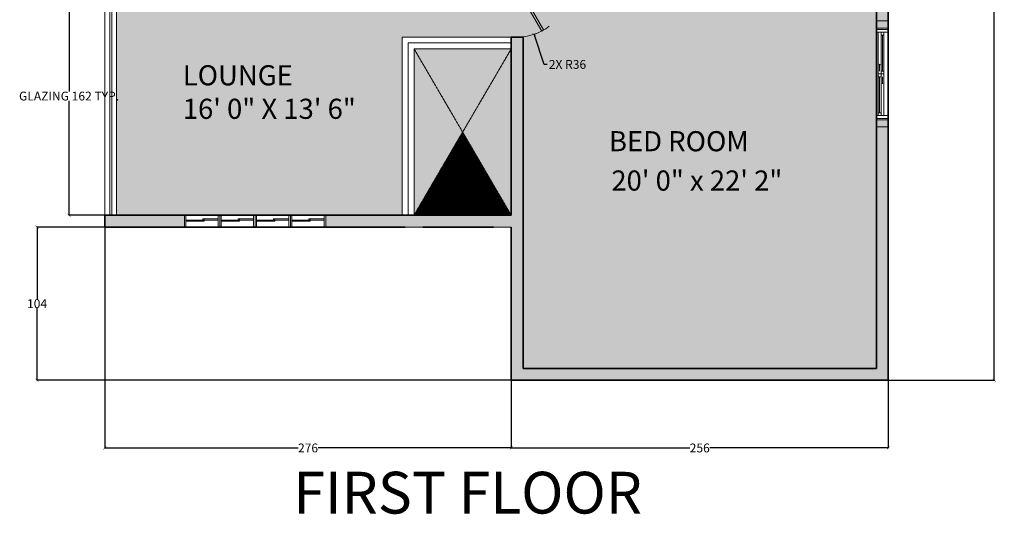
# Model space of a CAD drawing. Units: inches. Extents: x 1704 to 6393, y -157 to 1172.
# Tile 117 of 122: x 4377 to 5046, y 47 to 382. Entities that reach past the tile are written whole.
import ezdxf

# ---------------------------------------------------------------- set-up
doc = ezdxf.new("R2010")
doc.units = ezdxf.units.IN
doc.header["$MEASUREMENT"] = 0
doc.linetypes.add('ACAD_ISO02W100', pattern=[15, 12, -3])
doc.linetypes.add('HIDDEN', pattern=[0.375, 0.25, -0.125])
for name, color, linetype, lineweight in [('A-ANNO-DIMS', 7, 'Continuous', 13), ('A-ANNO-TEXT', 7, 'Continuous', 25), ('A-AREA-IDEN', 7, 'Continuous', 18), ('A-FLOR-OPEN-HIDN', 8, 'HIDDEN', 13), ('A-WALL-OVHD', 8, 'ACAD_ISO02W100', 13), ('A-WALL-PATT', 7, 'Continuous', 13), ('DOORS', 160, 'Continuous', 18), ('GLASS PANEL FASADE', 4, 'Continuous', 18), ('WALLS', 7, 'Continuous', 35), ('WINDOWS', 2, 'Continuous', 18)]:
    doc.layers.add(name, color=color, linetype=linetype, lineweight=lineweight)
doc.layers.add('A-FLOR-PATT', color=7, linetype='Continuous', lineweight=13, true_color=0xf2f2f2)
doc.styles.get("Standard").update_dxf_attribs({"font": 'arial.ttf'})
doc.dimstyles.get("Standard").update_dxf_attribs({"dimtxt": 6, "dimasz": 2, "dimexe": 0.18, "dimexo": 0.0625, "dimgap": 0.09, "dimtad": 0, "dimtih": 1, "dimtoh": 1, "dimdec": 1, "dimzin": 0, "dimdsep": 46, "dimlunit": 3, "dimtxsty": 'Standard', "dimblk": 'ARCHTICK', "dimcen": 0.09, "dimadec": 0, "dimazin": 0, "dimtfac": 1, "dimtdec": 1, "dimtofl": 0, "dimtmove": 0, "dimatfit": 3, "dimfxl": 1, "dimtolj": 1, "dimtzin": 0, "dimarcsym": 0})

# ---------------------------------------------------------------- blocks, each defined once
blk = doc.blocks.new('Door - Left Hung 36 in.')
blk.add_lwpolyline([(0.75, -1.3), (0, 0), (31.18, 18), (31.93, 16.7)], close=True)
blk.add_arc((0, 0), 36, 0, 37.31013)
blk = doc.blocks.new('WIN-SLIDER-72')
for p, q in [((0, 72), (0, 0)), ((0, 72), (8, 72)), ((0, 67.23), (8, 67.23)), ((8, 66.25), (8, 72)), ((1.17, 36), (1.17, 64.3)), ((3.12, 37.95), (3.12, 62.35)), ((4.1, 37.95), (4.1, 62.35)), ((5.07, 37.95), (5.07, 62.35)), ((8, 7.7), (8, 64.3)), ((2.14, 37.95), (2.14, 42.14)), ((1.17, 9.65), (1.17, 34.05)), ((2.14, 9.65), (2.14, 34.05)), ((3.12, 9.65), (3.12, 34.05)), ((4.1, 34.05), (4.1, 29.86)), ((5.07, 36), (5.07, 7.7)), ((0, 4.77), (8, 4.77)), ((8, 5.75), (8, 0)), ((0, 0), (8, 0))]:
    blk.add_line(p, q)
for points in [[(8, 64.3), (8, 66.25), (0, 66.25), (0, 64.3)], [(5.07, 62.35), (5.07, 64.3), (3.12, 64.3), (3.12, 62.35)], [(2.14, 42.65), (1.85, 42.14), (2.44, 42.14)], [(3.12, 34.05), (3.12, 36), (1.17, 36), (1.17, 34.05)], [(5.07, 36), (5.07, 37.95), (3.12, 37.95), (3.12, 36)], [(4.1, 29.35), (3.8, 29.86), (4.39, 29.86)], [(8, 7.7), (8, 5.75), (0, 5.75), (0, 7.7)], [(3.12, 7.7), (3.12, 9.65), (1.17, 9.65), (1.17, 7.7)]]:
    blk.add_lwpolyline(points, close=True)
blk = doc.blocks.new('GLAZ-FOUR-PANEL-96')
for p, q in [((96, 8), (0, 8)), ((0, 8), (0, 0)), ((1, 8), (1, 0)), ((23, 8), (23, 0)), ((24, 8), (24, 0)), ((25, 8), (25, 0)), ((47, 8), (47, 0)), ((48, 8), (48, 0)), ((49, 8), (49, 0)), ((71, 8), (71, 0)), ((72, 8), (72, 0)), ((73, 8), (73, 0)), ((95, 0), (95, 8)), ((96, 0), (96, 8)), ((12.51, 4.77), (1, 4.77)), ((1, 4), (12.51, 4)), ((12.51, 4.77), (12.51, 5.55)), ((12.51, 5.55), (23, 5.55)), ((12.51, 4), (12.51, 4.77)), ((12.51, 4.77), (23, 4.77)), ((12.51, 4), (13.51, 4)), ((13.51, 4), (13.51, 5.55)), ((36.51, 4.77), (25, 4.77)), ((25, 4), (36.51, 4)), ((36.51, 4.77), (36.51, 5.55)), ((36.51, 5.55), (47, 5.55)), ((36.51, 4), (36.51, 4.77)), ((36.51, 4.77), (47, 4.77)), ((36.51, 4), (37.51, 4)), ((37.51, 4), (37.51, 5.55)), ((60.51, 4.77), (49, 4.77)), ((49, 4), (60.51, 4)), ((60.51, 4.77), (60.51, 5.55)), ((60.51, 5.55), (71, 5.55)), ((60.51, 4), (60.51, 4.77)), ((60.51, 4.77), (71, 4.77)), ((60.51, 4), (61.51, 4)), ((61.51, 4), (61.51, 5.55)), ((84.51, 4.77), (73, 4.77)), ((73, 4), (84.51, 4)), ((84.51, 4.77), (84.51, 5.55)), ((84.51, 5.55), (95, 5.55)), ((84.51, 4), (84.51, 4.77)), ((84.51, 4.77), (95, 4.77)), ((84.51, 4), (85.51, 4)), ((85.51, 4), (85.51, 5.55)), ((0, 0), (96, 0))]:
    blk.add_line(p, q)
blk = doc.blocks.new('GLAZ-PANEL-162')
for p, q in [((3.3, 0), (3.3, 162)), ((4.7, 0), (4.7, 162))]:
    blk.add_line(p, q)
blk.add_lwpolyline([(8, 0), (0, 0), (0, 162), (8, 162)], close=True)
blk = doc.blocks.new('_ArchTick')
at = {"color": 0, "linetype": 'ByBlock', "const_width": 0.15}
blk.add_lwpolyline([(-0.5, -0.5), (0.5, 0.5)], dxfattribs=at)
blk = doc.blocks.new('*D48')
at = {"layer": 'A-ANNO-DIMS', "color": 0, "lineweight": -2, "transparency": 16777216}
for p, q in [((4435.24, 411.62), (4410.82, 411.62)), ((4411, 411.62), (4411, 333.82)), ((4411, 249.62), (4411, 327.43)), ((4435.24, 249.62), (4410.82, 249.62))]:
    blk.add_line(p, q, dxfattribs=at)
at = {"layer": 'Defpoints', "color": 0, "lineweight": -3, "transparency": 16777216}
for p in [(4411, 411.62), (4435.3, 411.62), (4435.3, 249.62)]:
    blk.add_point(p, dxfattribs=at)
at = {"layer": 'A-ANNO-DIMS', "color": 0, "lineweight": -2, "transparency": 16777216, "xscale": 2, "yscale": 2, "zscale": 2}
for p, rotation in [((4411, 411.62), 90), ((4411, 249.62), 270)]:
    blk.add_blockref('_ArchTick', p, dxfattribs=dict(at, rotation=rotation))
at = {"layer": 'A-ANNO-DIMS', "color": 0, "transparency": 16777216, "insert": (4411, 330.62), "char_height": 6, "attachment_point": 5}
blk.add_mtext('\\A1;GLAZING 162 TYP.', dxfattribs=at)
blk = doc.blocks.new('*D108')
at = {"layer": 'A-ANNO-DIMS', "color": 0, "lineweight": -2, "transparency": 16777216}
for p, q in [((4967.36, 942.62), (5039.48, 942.62)), ((5039.3, 942.62), (5039.3, 543.28)), ((5039.3, 137.62), (5039.3, 536.97)), ((4967.36, 137.62), (5039.48, 137.62))]:
    blk.add_line(p, q, dxfattribs=at)
at = {"layer": 'Defpoints', "color": 0, "lineweight": -3, "transparency": 16777216}
for p in [(4967.3, 942.62), (5039.3, 942.62), (4967.3, 137.62)]:
    blk.add_point(p, dxfattribs=at)
at = {"layer": 'A-ANNO-DIMS', "color": 0, "lineweight": -2, "transparency": 16777216, "xscale": 2, "yscale": 2, "zscale": 2}
for p, rotation in [((5039.3, 942.62), 90), ((5039.3, 137.62), 270)]:
    blk.add_blockref('_ArchTick', p, dxfattribs=dict(at, rotation=rotation))
at = {"layer": 'A-ANNO-DIMS', "color": 0, "transparency": 16777216, "insert": (5039.3, 540.12), "char_height": 6, "attachment_point": 5}
blk.add_mtext('\\A1;805', dxfattribs=at)
blk = doc.blocks.new('*D109')
at = {"layer": 'A-ANNO-DIMS', "color": 0, "lineweight": -2, "transparency": 16777216}
for p, q in [((4435.31, 241.56), (4435.31, 91.44)), ((4711.3, 241.56), (4711.3, 91.44)), ((4435.31, 91.62), (4566.54, 91.62)), ((4711.3, 91.62), (4580.07, 91.62))]:
    blk.add_line(p, q, dxfattribs=at)
at = {"layer": 'Defpoints', "color": 0, "lineweight": -3, "transparency": 16777216}
for p in [(4435.31, 241.62), (4711.3, 241.62), (4711.3, 91.62)]:
    blk.add_point(p, dxfattribs=at)
at = {"layer": 'A-ANNO-DIMS', "color": 0, "lineweight": -2, "transparency": 16777216, "xscale": 2, "yscale": 2, "zscale": 2, "rotation": 180}
blk.add_blockref('_ArchTick', (4435.31, 91.62), dxfattribs=at)
at = {"layer": 'A-ANNO-DIMS', "color": 0, "lineweight": -2, "transparency": 16777216, "xscale": 2, "yscale": 2, "zscale": 2}
blk.add_blockref('_ArchTick', (4711.3, 91.62), dxfattribs=at)
at = {"layer": 'A-ANNO-DIMS', "color": 0, "transparency": 16777216, "insert": (4573.31, 91.62), "char_height": 6, "attachment_point": 5}
blk.add_mtext('\\A1;276', dxfattribs=at)
blk = doc.blocks.new('*D110')
at = {"layer": 'A-ANNO-DIMS', "color": 0, "lineweight": -2, "transparency": 16777216}
for p, q in [((4711.3, 137.56), (4711.3, 91.44)), ((4967.3, 137.56), (4967.3, 91.44)), ((4711.3, 91.62), (4832.53, 91.62)), ((4967.3, 91.62), (4846.07, 91.62))]:
    blk.add_line(p, q, dxfattribs=at)
at = {"layer": 'Defpoints', "color": 0, "lineweight": -3, "transparency": 16777216}
for p in [(4711.3, 137.62), (4967.3, 137.62), (4967.3, 91.62)]:
    blk.add_point(p, dxfattribs=at)
at = {"layer": 'A-ANNO-DIMS', "color": 0, "lineweight": -2, "transparency": 16777216, "xscale": 2, "yscale": 2, "zscale": 2, "rotation": 180}
blk.add_blockref('_ArchTick', (4711.3, 91.62), dxfattribs=at)
at = {"layer": 'A-ANNO-DIMS', "color": 0, "lineweight": -2, "transparency": 16777216, "xscale": 2, "yscale": 2, "zscale": 2}
blk.add_blockref('_ArchTick', (4967.3, 91.62), dxfattribs=at)
at = {"layer": 'A-ANNO-DIMS', "color": 0, "transparency": 16777216, "insert": (4839.3, 91.62), "char_height": 6, "attachment_point": 5}
blk.add_mtext('\\A1;256', dxfattribs=at)
blk = doc.blocks.new('*D111')
at = {"layer": 'A-ANNO-DIMS', "color": 0, "lineweight": -2, "transparency": 16777216}
for p, q in [((4435.25, 241.62), (4389.12, 241.62)), ((4389.3, 241.62), (4389.3, 192.78)), ((4389.3, 137.62), (4389.3, 186.47)), ((4711.24, 137.62), (4389.12, 137.62))]:
    blk.add_line(p, q, dxfattribs=at)
at = {"layer": 'Defpoints', "color": 0, "lineweight": -3, "transparency": 16777216}
for p in [(4435.31, 241.62), (4389.3, 137.62), (4711.3, 137.62)]:
    blk.add_point(p, dxfattribs=at)
at = {"layer": 'A-ANNO-DIMS', "color": 0, "lineweight": -2, "transparency": 16777216, "xscale": 2, "yscale": 2, "zscale": 2}
for p, rotation in [((4389.3, 241.62), 90), ((4389.3, 137.62), 270)]:
    blk.add_blockref('_ArchTick', p, dxfattribs=dict(at, rotation=rotation))
at = {"layer": 'A-ANNO-DIMS', "color": 0, "transparency": 16777216, "insert": (4389.3, 189.62), "char_height": 6, "attachment_point": 5}
blk.add_mtext('\\A1;104', dxfattribs=at)
blk = doc.blocks.new('*D138')
at = {"layer": 'A-ANNO-DIMS', "color": 0, "lineweight": -2, "transparency": 16777216}
for p, q in [((4715.21, 406.69), (4715.39, 406.69)), ((4715.3, 406.6), (4715.3, 406.78)), ((4733.73, 352.12), (4726.82, 372.59)), ((4735.73, 352.12), (4733.73, 352.12))]:
    blk.add_line(p, q, dxfattribs=at)
at = {"layer": 'Defpoints', "color": 0, "lineweight": -3, "transparency": 16777216}
for p in [(4715.3, 406.69), (4726.82, 372.59)]:
    blk.add_point(p, dxfattribs=at)
at = {"layer": 'A-ANNO-DIMS', "color": 0, "lineweight": -2, "transparency": 16777216, "xscale": 2, "yscale": 2, "zscale": 2, "rotation": 108.6557587224779}
blk.add_blockref('_ArchTick', (4726.82, 372.59), dxfattribs=at)
at = {"layer": 'A-ANNO-DIMS', "color": 0, "transparency": 16777216, "insert": (4749.48, 352.12), "char_height": 6, "attachment_point": 5}
blk.add_mtext('\\A1;2X R36', dxfattribs=at)

msp = doc.modelspace()

# ---------------------------------------------------------------- hatches: boundary and pattern name
at = {"layer": 'A-FLOR-PATT', "transparency": 33554516}
h = msp.add_hatch(color=256, dxfattribs=at)
h.dxf.hatch_style = 1
h.paths.add_polyline_path([(4859.3, 934.624), (4639.3, 934.624), (4639.3, 766.624), (4645.3, 766.624), (4645.3, 762.624), (4676.477, 780.624), (4677.227, 779.325), (4677.2, 779.309, -0.0929107), (4681.077, 766.624), (4687.3, 766.624), (4859.3, 766.624), (4859.3, 798.624), (4863.3, 798.624), (4863.3, 766.624), (4875.3, 766.624), (4959.3, 766.624), (4959.3, 834.624), (4923.217, 834.624, -0.0999534), (4920.567, 825.5), (4920.585, 825.49), (4920.085, 824.624), (4899.3, 836.624), (4899.3, 834.624), (4863.3, 834.624), (4859.3, 834.624)])
h.paths.add_polyline_path([(4631.3, 890.624), (4443.3, 890.624), (4443.3, 722.624), (4559.3, 722.624), (4559.3, 718.624), (4535.3, 718.624), (4535.3, 712.624), (4531.3, 712.624), (4532.383, 711.999), (4517.396, 686.04, 0.1210664), (4531.3, 682.624), (4535.3, 682.624), (4535.3, 609.624), (4631.3, 609.624), (4631.3, 718.624), (4595.3, 718.624), (4595.3, 722.624), (4631.3, 722.624), (4637.3, 722.624, -0.1140277), (4621.609, 726.711), (4621.593, 726.684), (4620.293, 727.435), (4638.3, 758.624), (4631.3, 758.624)])
h.paths.add_polyline_path([(4531.3, 712.624), (4527.3, 712.624), (4527.3, 718.624), (4443.3, 718.624), (4443.3, 609.624), (4527.3, 609.624), (4527.3, 682.891, -0.0872676), (4517.396, 686.04), (4517.383, 686.018), (4516.3, 686.643)], flags=17)
h.paths.add_polyline_path([(4631.3, 601.624), (4537.3, 510.624), (4631.3, 419.624)], flags=17)
h.paths.add_polyline_path([(4537.3, 510.624), (4443.3, 419.624), (4453.75, 419.624), (4617.46, 419.624), (4631.3, 419.624)], flags=17)
h.paths.add_polyline_path([(4443.3, 601.624), (4443.3, 419.624), (4537.3, 510.624)], flags=17)
h.paths.add_polyline_path([(4631.3, 601.624), (4443.3, 601.624), (4537.3, 510.624)], flags=17)
h.paths.add_polyline_path([(4637.3, 370.694), (4711.3, 370.694), (4715.3, 370.694, 0.1210664), (4731.986, 374.795), (4713.568, 406.694), (4711.3, 406.694), (4711.3, 419.624), (4712.3, 419.624), (4712.3, 613.124), (4720.3, 613.124), (4720.3, 592.624), (4782.3, 592.624), (4782.3, 657.624), (4720.3, 657.624), (4720.3, 637.124), (4712.3, 637.124), (4712.3, 662.624), (4787.3, 662.624), (4787.3, 654.624), (4787.3, 593.624), (4959.3, 593.624), (4959.3, 654.624), (4811.3, 654.624), (4811.3, 662.624), (4813.69, 662.624), (4813.69, 706.624), (4789.69, 706.624), (4789.69, 712.624), (4729.69, 712.624), (4729.69, 714.624), (4729.69, 758.624), (4681.3, 758.624), (4681.3, 762.624, 0.1210664), (4677.2, 779.309), (4645.3, 760.892), (4645.3, 758.624), (4638.3, 758.624), (4639.6, 757.873), (4621.609, 726.711, 0.1140277), (4637.3, 722.624), (4639.3, 722.624), (4639.3, 601.624), (4639.3, 419.624), (4639.3, 411.624), (4617.46, 411.624), (4453.75, 411.624), (4443.3, 411.624), (4443.3, 249.624), (4637.3, 249.624)])
h.paths.add_polyline_path([(4813.69, 758.624), (4790.69, 758.624), (4790.69, 714.624), (4813.69, 714.624)], flags=17)
h.paths.add_polyline_path([(4789.69, 758.624), (4780.69, 758.624), (4780.69, 714.624), (4789.69, 714.624)], flags=17)
h.paths.add_polyline_path([(4779.69, 758.624), (4770.69, 758.624), (4770.69, 714.624), (4779.69, 714.624)], flags=17)
h.paths.add_polyline_path([(4769.69, 758.624), (4760.69, 758.624), (4760.69, 714.624), (4769.69, 714.624)], flags=17)
h.paths.add_polyline_path([(4759.69, 758.624), (4750.69, 758.624), (4750.69, 714.624), (4759.69, 714.624)], flags=17)
h.paths.add_polyline_path([(4749.69, 758.624), (4740.69, 758.624), (4740.69, 714.624), (4749.69, 714.624)], flags=17)
h.paths.add_polyline_path([(4739.69, 758.624), (4730.69, 758.624), (4730.69, 714.624), (4739.69, 714.624)], flags=17)
h.paths.add_polyline_path([(4823.69, 758.624), (4814.69, 758.624), (4814.69, 714.624), (4823.69, 714.624)], flags=17)
h.paths.add_polyline_path([(4833.69, 758.624), (4824.69, 758.624), (4824.69, 714.624), (4833.69, 714.624)], flags=17)
h.paths.add_polyline_path([(4843.69, 758.624), (4834.69, 758.624), (4834.69, 714.624), (4843.69, 714.624)], flags=17)
h.paths.add_polyline_path([(4909.3, 706.624), (4894.69, 706.624), (4894.69, 662.624), (4909.3, 662.624)], flags=17)
h.paths.add_polyline_path([(4883.69, 706.624), (4874.69, 706.624), (4874.69, 662.624), (4883.69, 662.624)], flags=17)
h.paths.add_polyline_path([(4853.69, 706.624), (4844.69, 706.624), (4844.69, 662.624), (4853.69, 662.624)], flags=17)
h.paths.add_polyline_path([(4833.69, 706.624), (4824.69, 706.624), (4824.69, 662.624), (4833.69, 662.624)], flags=17)
h.paths.add_polyline_path([(4823.69, 706.624), (4814.69, 706.624), (4814.69, 662.624), (4823.69, 662.624)], flags=17)
h.paths.add_polyline_path([(4843.69, 706.624), (4834.69, 706.624), (4834.69, 662.624), (4843.69, 662.624)], flags=17)
h.paths.add_polyline_path([(4863.69, 706.624), (4854.69, 706.624), (4854.69, 662.624), (4863.69, 662.624)], flags=17)
h.paths.add_polyline_path([(4873.69, 706.624), (4864.69, 706.624), (4864.69, 662.624), (4873.69, 662.624)], flags=17)
h.paths.add_polyline_path([(4893.69, 706.624), (4884.69, 706.624), (4884.69, 662.624), (4893.69, 662.624)], flags=17)
h.paths.add_polyline_path([(4853.69, 758.624), (4844.69, 758.624), (4844.69, 714.624), (4853.69, 714.624)], flags=17)
h.paths.add_polyline_path([(4873.69, 758.624), (4864.69, 758.624), (4864.69, 714.624), (4873.69, 714.624)], flags=17)
h.paths.add_polyline_path([(4893.69, 758.624), (4884.69, 758.624), (4884.69, 714.624), (4893.69, 714.624)], flags=17)
h.paths.add_polyline_path([(4909.3, 758.624), (4894.69, 758.624), (4894.69, 714.624), (4909.3, 714.624)], flags=17)
h.paths.add_polyline_path([(4863.69, 758.624), (4854.69, 758.624), (4854.69, 714.624), (4863.69, 714.624)], flags=17)
h.paths.add_polyline_path([(4883.69, 758.624), (4874.69, 758.624), (4874.69, 714.624), (4883.69, 714.624)], flags=17)
h.paths.add_polyline_path([(4907.3, 712.624), (4813.69, 712.624), (4813.69, 708.624), (4907.3, 708.624)], flags=17)
at = {"layer": 'A-FLOR-PATT', "transparency": 33554511}
h = msp.add_hatch(color=256, dxfattribs=at)
h.dxf.hatch_style = 1
h.paths.add_polyline_path([(4860.3, 585.624), (4839.3, 585.624), (4720.3, 585.624), (4720.3, 466.624), (4766.3, 466.624), (4766.3, 462.624), (4720.3, 462.624), (4720.3, 419.624), (4766.3, 419.624), (4766.3, 415.624), (4767.05, 416.923), (4798.2, 398.938, 0.1210664), (4802.3, 415.624), (4802.3, 419.624), (4959.3, 419.624), (4959.3, 423.456), (4959.3, 424.757), (4959.3, 462.49), (4959.3, 463.791), (4959.3, 467.624), (4959.3, 543.32), (4864.3, 543.32), (4864.3, 462.624), (4802.3, 462.624), (4802.3, 466.624), (4860.3, 466.624)], flags=17)
h.paths.add_polyline_path([(4959.3, 411.624), (4802.077, 411.624, -0.0929107), (4798.2, 398.938), (4767.05, 416.923), (4766.3, 415.624), (4766.3, 411.624), (4719.3, 411.624), (4719.3, 406.694), (4711.3, 406.694), (4711.3, 419.624), (4712.3, 419.624), (4712.3, 613.124), (4720.3, 613.124), (4720.3, 592.624), (4782.3, 592.624), (4782.3, 657.624), (4720.3, 657.624), (4720.3, 637.124), (4712.3, 637.124), (4712.3, 662.624), (4787.3, 662.624), (4787.3, 654.624), (4787.3, 593.624), (4959.3, 593.624), (4959.3, 654.624), (4811.3, 654.624), (4811.3, 662.624), (4813.69, 662.624), (4813.69, 706.624), (4789.69, 706.624), (4789.69, 712.624), (4729.69, 712.624), (4729.69, 714.624), (4729.69, 758.624), (4681.3, 758.624), (4681.3, 766.624), (4687.3, 766.624), (4859.3, 766.624), (4859.3, 798.624), (4863.3, 798.624), (4863.3, 766.624), (4875.3, 766.624), (4959.3, 766.624), (4959.3, 834.624), (4923.3, 834.624), (4923.3, 838.624), (4959.3, 838.624), (4959.3, 892.32), (4863.3, 892.32), (4863.3, 838.624), (4899.3, 838.624), (4899.3, 834.624), (4863.3, 834.624), (4859.3, 834.624), (4859.3, 934.624), (4639.3, 934.624), (4639.3, 766.624), (4645.3, 766.624), (4645.3, 758.624), (4631.3, 758.624), (4631.3, 890.624), (4443.3, 890.624), (4443.3, 722.624), (4559.3, 722.624), (4559.3, 718.624), (4535.3, 718.624), (4535.3, 712.624), (4527.3, 712.624), (4527.3, 718.624), (4443.3, 718.624), (4443.3, 609.624), (4527.3, 609.624), (4527.3, 682.624), (4535.3, 682.624), (4535.3, 609.624), (4631.3, 609.624), (4631.3, 718.624), (4595.3, 718.624), (4595.3, 722.624), (4631.3, 722.624), (4639.3, 722.624), (4639.3, 601.624), (4639.3, 419.624), (4639.3, 411.624), (4617.46, 411.624), (4453.75, 411.624), (4443.3, 411.624), (4443.3, 249.624), (4637.3, 249.624), (4637.3, 370.694), (4711.3, 370.694), (4719.3, 370.694), (4719.3, 145.624), (4959.3, 145.624), (4959.3, 265.624)])
h.paths.add_polyline_path([(4645.3, 362.694), (4645.3, 249.624), (4678.295, 306.15)], flags=17)
h.paths.add_polyline_path([(4711.3, 362.694), (4645.3, 362.694), (4678.295, 306.15)], flags=17)
h.paths.add_polyline_path([(4711.3, 362.694), (4678.295, 306.15), (4711.279, 249.624), (4711.3, 249.624)], flags=17)
at = {"layer": 'A-FLOR-PATT', "transparency": 33554526}
h = msp.add_hatch(dxfattribs=at)
h.set_pattern_fill('ANSI31', color=256)
h.paths.add_polyline_path([(4678.295, 306.15), (4645.3, 249.624), (4651.3, 249.624), (4711.279, 249.624)])
at = {"layer": 'A-WALL-PATT'}
h = msp.add_hatch(color=256, dxfattribs=at)
h.dxf.hatch_style = 1
h.paths.add_polyline_path([(4967.3, 942.624), (4699.009, 942.624), (4699.009, 934.624), (4859.3, 934.624), (4859.3, 834.624), (4863.3, 834.624), (4899.3, 834.624), (4899.3, 838.624), (4863.3, 838.624), (4863.3, 934.624), (4959.3, 934.624), (4959.3, 901.624), (4959.3, 834.624), (4959.3, 766.624), (4863.3, 766.624), (4863.3, 798.624), (4859.3, 798.624), (4859.3, 766.624), (4687.3, 766.624), (4681.3, 766.624), (4681.3, 758.624), (4909.3, 758.624), (4909.3, 662.624), (4811.3, 662.624), (4811.3, 654.624), (4959.3, 654.624), (4959.3, 593.624), (4787.3, 593.624), (4787.3, 654.624), (4787.3, 662.624), (4712.3, 662.624), (4712.3, 637.124), (4720.3, 637.124), (4720.3, 657.624), (4782.3, 657.624), (4782.3, 592.624), (4720.3, 592.624), (4720.3, 613.124), (4712.3, 613.124), (4712.3, 419.624), (4711.3, 419.624), (4711.3, 406.694), (4719.3, 406.694), (4719.3, 411.624), (4766.3, 411.624), (4766.3, 419.624), (4720.3, 419.624), (4720.3, 462.624), (4766.3, 462.624), (4766.3, 466.624), (4720.3, 466.624), (4720.3, 585.624), (4839.3, 585.624), (4860.3, 585.624), (4860.3, 466.624), (4802.3, 466.624), (4802.3, 462.624), (4864.3, 462.624), (4864.3, 585.624), (4959.3, 585.624), (4959.3, 542.624), (4959.3, 467.624), (4967.3, 467.624), (4967.3, 559.624), (4993.3, 559.624), (4993.3, 567.435), (4991.3, 567.435), (4991.3, 561.624), (4967.3, 561.624), (4967.3, 613.624), (4991.3, 613.624), (4991.3, 605.789), (4993.3, 605.789), (4993.3, 615.624), (4967.3, 615.624), (4967.3, 654.624), (4967.3, 662.624), (4959.3, 662.624), (4913.3, 662.624), (4913.3, 758.624), (4959.3, 758.624), (4959.3, 692.624), (4967.3, 692.624), (4967.3, 759.624), (4993.3, 759.624), (4993.3, 801.624), (4967.3, 801.624)])
h.paths.add_polyline_path([(4967.3, 799.624), (4991.3, 799.624), (4991.3, 763.624), (4967.3, 763.624)], flags=16)
h.paths.add_polyline_path([(4443.3, 718.624), (4527.3, 718.624), (4527.3, 712.624), (4535.3, 712.624), (4535.3, 718.624), (4559.3, 718.624), (4559.3, 722.624), (4443.3, 722.624), (4435.3, 722.624), (4435.3, 601.624), (4443.3, 601.624), (4639.3, 601.624), (4639.3, 722.624), (4631.3, 722.624), (4595.3, 722.624), (4595.3, 718.624), (4631.3, 718.624), (4631.3, 609.624), (4535.3, 609.624), (4535.3, 682.624), (4527.3, 682.624), (4527.3, 609.624), (4443.3, 609.624)])
h.paths.add_polyline_path([(4443.3, 890.624), (4489.3, 890.624), (4489.3, 898.624), (4443.3, 898.624), (4443.3, 934.624), (4455.446, 934.624), (4455.446, 942.624), (4435.3, 942.624), (4435.3, 794.624), (4443.3, 794.624)])
h.paths.add_polyline_path([(4639.3, 934.624), (4651.009, 934.624), (4651.009, 942.624), (4635.3, 942.624), (4619.155, 942.624), (4619.155, 934.624), (4631.3, 934.624), (4631.3, 898.624), (4585.3, 898.624), (4585.3, 890.624), (4631.3, 890.624), (4631.3, 758.624), (4645.3, 758.624), (4645.3, 766.624), (4639.3, 766.624)])
h.paths.add_polyline_path([(4967.3, 265.624), (4967.3, 309.624), (4959.3, 309.624), (4959.3, 265.624), (4959.3, 145.624), (4719.3, 145.624), (4719.3, 370.694), (4711.3, 370.694), (4711.3, 249.624), (4699.3, 249.624), (4651.3, 249.624), (4639.3, 249.624), (4585.307, 249.624), (4585.307, 241.624), (4639.3, 241.624), (4651.3, 241.624), (4699.3, 241.624), (4711.3, 241.624), (4711.3, 137.624), (4719.3, 137.624), (4959.3, 137.624), (4967.3, 137.624)])
h.paths.add_polyline_path([(4489.307, 249.624), (4435.313, 249.624), (4435.313, 241.624), (4489.307, 241.624)])
h.paths.add_polyline_path([(4967.3, 419.624), (4959.3, 419.624), (4802.3, 419.624), (4802.3, 411.624), (4959.3, 411.624), (4959.3, 381.624), (4967.3, 381.624)])
h.paths.add_polyline_path([(4967.3, 381.624), (4959.3, 381.624), (4959.3, 376.851), (4967.3, 376.851)])
h.paths.add_polyline_path([(4967.3, 314.396), (4959.3, 314.396), (4959.3, 309.624), (4967.3, 309.624)], flags=17)
h.paths.add_polyline_path([(4959.3, 838.624), (4923.3, 838.624), (4923.3, 834.624), (4959.3, 834.624)], flags=17)

# ---------------------------------------------------------------- linework, layer by layer
at = {"layer": 'A-FLOR-OPEN-HIDN'}
for p, q in [((4645.3, 249.624), (4711.3, 362.694)), ((4711.181, 249.792), (4645.3, 362.694))]:
    msp.add_line(p, q, dxfattribs=at)
at = {"layer": 'A-WALL-OVHD'}
for p, q in [((4639.3, 249.624), (4651.3, 249.624)), ((4699.3, 249.624), (4711.3, 249.624)), ((4639.3, 241.624), (4651.3, 241.624)), ((4699.3, 241.624), (4711.3, 241.624))]:
    msp.add_line(p, q, dxfattribs=at)
at = {"layer": 'GLASS PANEL FASADE'}
for p, q in [((4637.3, 370.694), (4711.3, 370.694)), ((4637.3, 249.624), (4637.3, 370.694)), ((4641.3, 249.624), (4641.3, 366.694)), ((4711.3, 366.694), (4641.3, 366.694)), ((4645.3, 249.624), (4645.3, 362.694)), ((4645.3, 362.694), (4711.3, 362.694))]:
    msp.add_line(p, q, dxfattribs=at)
at = {"layer": 'WALLS'}
for p, q in [((4967.3, 265.624), (4967.3, 559.624)), ((4959.3, 265.624), (4959.3, 411.624)), ((4959.3, 375.624), (4959.3, 411.624)), ((4711.3, 249.624), (4711.3, 370.694)), ((4711.3, 370.694), (4719.3, 370.694)), ((4719.3, 145.624), (4719.3, 370.694)), ((4959.3, 317.624), (4959.3, 373.624)), ((4959.3, 145.624), (4959.3, 265.624)), ((4967.3, 137.624), (4967.3, 265.624)), ((4711.3, 249.624), (4435.3, 249.624)), ((4435.313, 241.624), (4435.3, 249.624)), ((4651.3, 249.624), (4699.3, 249.624)), ((4639.3, 241.624), (4435.313, 241.624)), ((4651.3, 241.624), (4699.3, 241.624)), ((4711.3, 137.624), (4711.3, 241.624)), ((4959.3, 145.624), (4719.3, 145.624)), ((4719.3, 137.624), (4711.3, 137.624)), ((4959.3, 137.624), (4719.3, 137.624)), ((4959.3, 137.624), (4967.3, 137.624))]:
    msp.add_line(p, q, dxfattribs=at)

# ---------------------------------------------------------------- block references
at = {"layer": 'DOORS', "rotation": 270}
msp.add_blockref('Door - Left Hung 36 in.', (4715.3, 406.694), dxfattribs=at)
at = {"layer": 'GLASS PANEL FASADE'}
for name, p in [('GLAZ-PANEL-162', (4435.301, 249.624)), ('GLAZ-FOUR-PANEL-96', (4489.307, 241.624))]:
    msp.add_blockref(name, p, dxfattribs=at)
at = {"layer": 'WINDOWS'}
msp.add_blockref('WIN-SLIDER-72', (4959.301, 309.624), dxfattribs=at)

# ---------------------------------------------------------------- texts
at = {"layer": 'A-ANNO-DIMS'}
for s, p in [('16\' 0" X 13\' 6"', (4488.242, 315.142)), ('20\' 0" x 22\' 2"', (4779.271, 266.415))]:
    msp.add_text(s, height=13.6672, dxfattribs=at).set_placement(p)
at = {"layer": 'A-ANNO-TEXT'}
msp.add_text('FIRST FLOOR', height=28.38733, dxfattribs=at).set_placement((4563.355, 47.052))
at = {"layer": 'A-AREA-IDEN'}
for s, p in [('LOUNGE', (4488.242, 337.904)), (' BED ROOM', (4773.461, 293.122))]:
    msp.add_text(s, height=13.6672, dxfattribs=at).set_placement(p)

# ---------------------------------------------------------------- dimensions: what is measured, and where the dimension line sits
at = {"layer": 'A-ANNO-DIMS'}
for base, p1, p2, picture, middle in [((5039.3, 942.624), (4967.3, 137.624), (4967.3, 942.624), '*D108', (5039.3, 540.124)), ((4389.3, 137.624), (4435.313, 241.624), (4711.3, 137.624), '*D111', (4389.3, 189.624))]:
    dim = msp.add_linear_dim(base=base, p1=p1, p2=p2, angle=90, dimstyle='Standard', override={"dimdec": 0, "dimlfac": 1, "dimrnd": 0, "dimzin": 0, "dimdsep": 46, "dimlunit": 2}, dxfattribs=at)
    dim.commit()
    dim.dimension.update_dxf_attribs({"geometry": picture, "text_midpoint": middle})
dim = msp.add_linear_dim(base=(4411, 411.624), p1=(4435.3, 249.624), p2=(4435.3, 411.624), angle=90, text='GLAZING <> TYP.', dimstyle='Standard', override={"dimdec": 0, "dimlfac": 1, "dimrnd": 0, "dimzin": 0, "dimdsep": 46, "dimlunit": 2}, dxfattribs=at)
dim.commit()
dim.dimension.update_dxf_attribs({"geometry": '*D48', "text_midpoint": (4411, 330.624)})
dim = msp.add_radius_dim(center=(4715.3, 406.694), mpoint=(4726.816, 372.586), text='2X <>', dimstyle='Standard', override={"dimdec": 0, "dimlfac": 1, "dimrnd": 0, "dimzin": 0, "dimdsep": 46, "dimlunit": 2}, dxfattribs=at)
dim.commit()
dim.dimension.update_dxf_attribs({"geometry": '*D138', "text_midpoint": (4749.479, 352.121), "dimtype": 164})
for base, p1, p2, picture, middle in [((4711.3, 91.624), (4435.313, 241.624), (4711.3, 241.624), '*D109', (4573.307, 91.624)), ((4967.3, 91.624), (4711.3, 137.624), (4967.3, 137.624), '*D110', (4839.3, 91.624))]:
    dim = msp.add_linear_dim(base=base, p1=p1, p2=p2, dimstyle='Standard', override={"dimdec": 0, "dimlfac": 1, "dimrnd": 0, "dimzin": 0, "dimdsep": 46, "dimlunit": 2}, dxfattribs=at)
    dim.commit()
    dim.dimension.update_dxf_attribs({"geometry": picture, "text_midpoint": middle})

doc.saveas('drawing.dxf')
